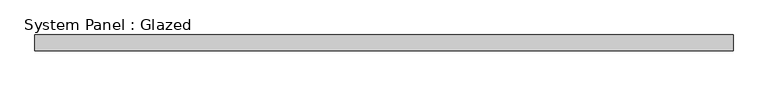
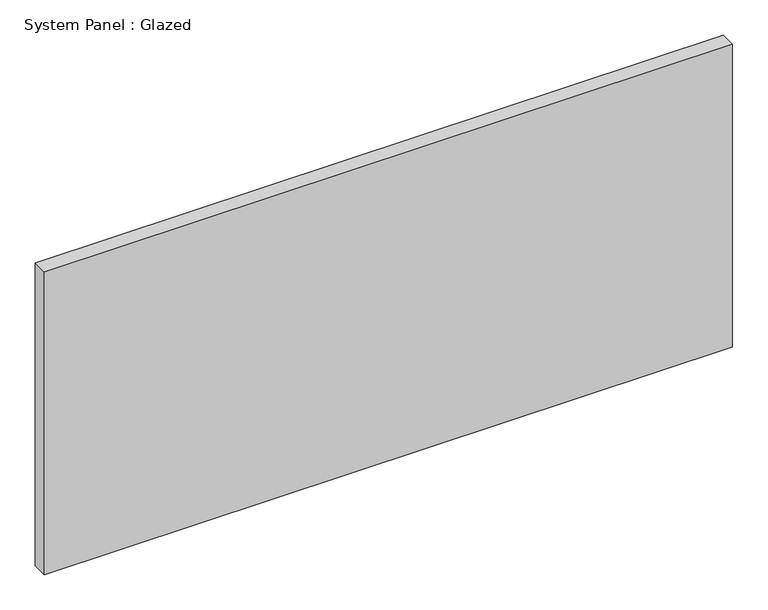
"""IFC4 building model written with IfcOpenShell, lengths in millimetres: plate geometry, System Panel : Glazed."""

from ifc_helpers import new_model, si_unit, origin, origin_with_axes, place, context, project, spatial, polyline, outline, extrude, source, transform, mapped, element, save


def system_panel_glazed_06acdacc(model_context):
    return source(origin(), model_context, "Body", "SweptSolid", [
        extrude(outline(polyline([(561.975, 19.05), (-561.975, 19.05), (-561.975, 44.45), (561.975, 44.45), (561.975, 19.05)])), origin_with_axes(), (0.0, 0.0, 1.0), 522.8166667),
    ])


if __name__ == "__main__":
    model = new_model("IFC4")
    model_context = context("Model", 3, world=origin())
    ifc_project = project(units=[si_unit("LENGTHUNIT", "METRE", prefix="MILLI")], contexts=[model_context])
    site = spatial("IfcSite", under=ifc_project)
    building = spatial("IfcBuilding", under=site)
    placement = place(None, origin())
    system_panel_glazed_shape = system_panel_glazed_06acdacc(model_context)
    element("IfcPlate", 1, ObjectType="System Panel : Glazed", at=placement, inside=building, context=model_context, shape_type="MappedRepresentation", body=[
        mapped(system_panel_glazed_shape, transform((0.0, 0.0, 0.0), x_axis=(1.0, 0.0, 0.0), y_axis=(0.0, 1.0, 0.0), z_axis=(0.0, 0.0, 1.0))),
    ])
    save(model, "model.ifc")

# Revit data of these elements
# Type "System Panel : Glazed"
#   Construction Type Id = "GSP4R"
#   Analytic Construction = "1/8 in Pilkington single glazing"
#   Visual Light Transmittance = 0.9
#   Solar Heat Gain Coefficient = 0.86
#   Heat Transfer Coefficient (U) = 1.18115 BTU/(h·ft²·°F)
#   Define Thermal Properties by = 1
# Element 1 (IfcPlate, "System Panel : Glazed")
#   Materials on its faces: "Glass"
# Materials
#   "Glass": class "Glass", colour RGB 0 128 192, transparency 0.75, Description = "Soda Lime Glass", Cost = 0
